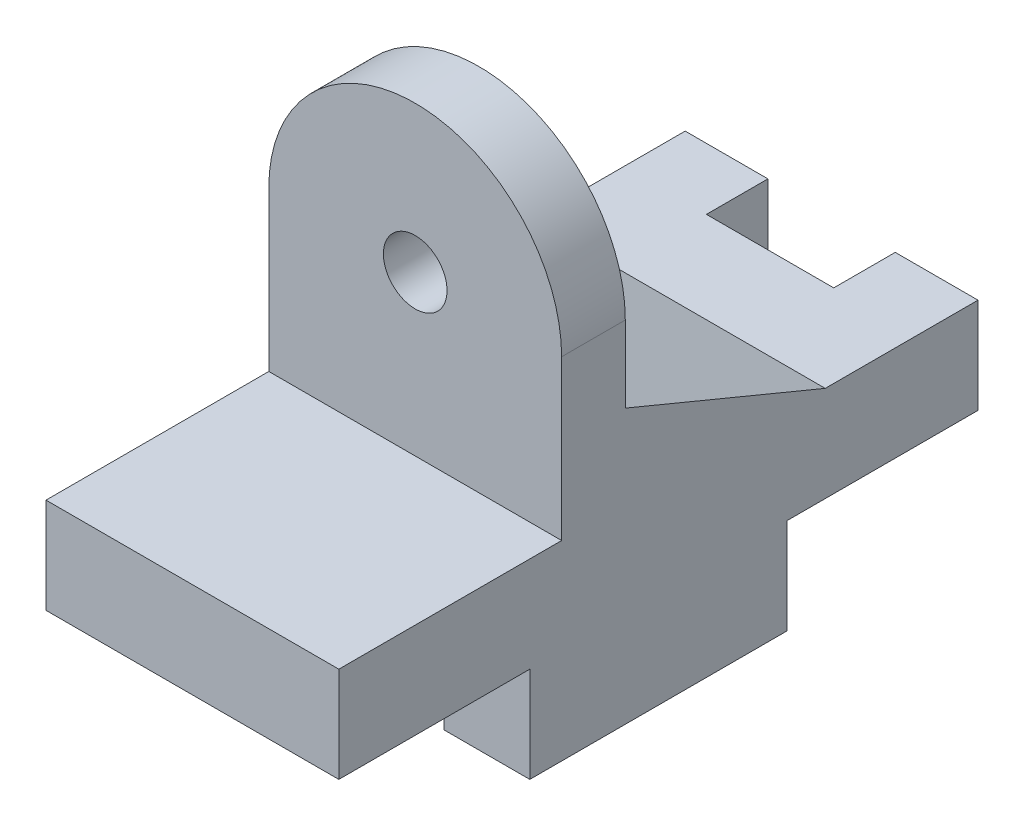
ISO-10303-21;
HEADER;
FILE_DESCRIPTION(('STEP AP214'),'2;1');
FILE_NAME('part.step','',(''),(''),'','','');
FILE_SCHEMA(('AUTOMOTIVE_DESIGN { 1 0 10303 214 1 1 1 1 }'));
ENDSEC;
DATA;
#1=APPLICATION_CONTEXT('core data for automotive mechanical design processes');
#2=APPLICATION_PROTOCOL_DEFINITION('international standard','automotive_design',2000,#1);
#3=PRODUCT_CONTEXT('',#1,'mechanical');
#4=PRODUCT('Part','Part','',(#3));
#5=PRODUCT_RELATED_PRODUCT_CATEGORY('part','',(#4));
#6=PRODUCT_DEFINITION_FORMATION('','',#4);
#7=PRODUCT_DEFINITION_CONTEXT('part definition',#1,'design');
#8=PRODUCT_DEFINITION('design','',#6,#7);
#9=PRODUCT_DEFINITION_SHAPE('','',#8);
#10=(LENGTH_UNIT() NAMED_UNIT(*) SI_UNIT(.MILLI.,.METRE.));
#11=(NAMED_UNIT(*) PLANE_ANGLE_UNIT() SI_UNIT($,.RADIAN.));
#12=(NAMED_UNIT(*) SI_UNIT($,.STERADIAN.) SOLID_ANGLE_UNIT());
#13=UNCERTAINTY_MEASURE_WITH_UNIT(LENGTH_MEASURE(1.E-05),#10,'distance_accuracy_value','');
#14=(GEOMETRIC_REPRESENTATION_CONTEXT(3) GLOBAL_UNCERTAINTY_ASSIGNED_CONTEXT((#13)) GLOBAL_UNIT_ASSIGNED_CONTEXT((#10,
#11,#12)) REPRESENTATION_CONTEXT('',''));
#15=CARTESIAN_POINT('',(0.,0.,0.));
#16=DIRECTION('',(0.,0.,1.));
#17=DIRECTION('',(1.,0.,0.));
#18=AXIS2_PLACEMENT_3D('',#15,#16,#17);
#19=CARTESIAN_POINT('',(46.,-15.,20.2023099235515));
#20=DIRECTION('',(0.,0.,-1.));
#21=DIRECTION('',(0.,1.,0.));
#22=AXIS2_PLACEMENT_3D('',#19,#20,#21);
#23=PLANE('',#22);
#24=DIRECTION('',(-1.,0.,0.));
#25=VECTOR('',#24,1.);
#26=CARTESIAN_POINT('',(46.,-30.,20.2023099235515));
#27=LINE('',#26,#25);
#28=CARTESIAN_POINT('',(13.5,-30.,20.2023099235515));
#29=VERTEX_POINT('',#28);
#30=CARTESIAN_POINT('',(0.,-30.,20.2023099235515));
#31=VERTEX_POINT('',#30);
#32=EDGE_CURVE('E220',#29,#31,#27,.T.);
#33=ORIENTED_EDGE('',*,*,#32,.F.);
#34=DIRECTION('',(0.,1.,0.));
#35=VECTOR('',#34,1.);
#36=CARTESIAN_POINT('',(13.5,-15.,20.2023099235515));
#37=LINE('',#36,#35);
#38=CARTESIAN_POINT('',(13.5,-15.,20.2023099235515));
#39=VERTEX_POINT('',#38);
#40=EDGE_CURVE('E346',#29,#39,#37,.T.);
#41=ORIENTED_EDGE('',*,*,#40,.T.);
#42=DIRECTION('',(-1.,0.,0.));
#43=VECTOR('',#42,1.);
#44=CARTESIAN_POINT('',(46.,-15.,20.2023099235515));
#45=LINE('',#44,#43);
#46=CARTESIAN_POINT('',(0.,-15.,20.2023099235515));
#47=VERTEX_POINT('',#46);
#48=EDGE_CURVE('E221',#39,#47,#45,.T.);
#49=ORIENTED_EDGE('',*,*,#48,.T.);
#50=DIRECTION('',(0.,-1.,0.));
#51=VECTOR('',#50,1.);
#52=CARTESIAN_POINT('',(0.,-15.,20.2023099235515));
#53=LINE('',#52,#51);
#54=EDGE_CURVE('E270',#47,#31,#53,.T.);
#55=ORIENTED_EDGE('',*,*,#54,.T.);
#56=EDGE_LOOP('',(#33,#41,#49,#55));
#57=FACE_BOUND('',#56,.T.);
#58=ADVANCED_FACE('F41',(#57),#23,.F.);
#59=CARTESIAN_POINT('',(46.,-30.,-20.2023099235515));
#60=DIRECTION('',(0.,1.,0.));
#61=DIRECTION('',(0.,0.,1.));
#62=AXIS2_PLACEMENT_3D('',#59,#60,#61);
#63=PLANE('',#62);
#64=DIRECTION('',(-1.,0.,0.));
#65=VECTOR('',#64,1.);
#66=CARTESIAN_POINT('',(46.,-30.,-20.2023099235515));
#67=LINE('',#66,#65);
#68=CARTESIAN_POINT('',(13.5,-30.,-20.2023099235515));
#69=VERTEX_POINT('',#68);
#70=CARTESIAN_POINT('',(0.,-30.,-20.2023099235515));
#71=VERTEX_POINT('',#70);
#72=EDGE_CURVE('E209',#69,#71,#67,.T.);
#73=ORIENTED_EDGE('',*,*,#72,.F.);
#74=DIRECTION('',(0.,0.,1.));
#75=VECTOR('',#74,1.);
#76=CARTESIAN_POINT('',(13.5,-30.,-20.2023099235515));
#77=LINE('',#76,#75);
#78=EDGE_CURVE('E351',#69,#29,#77,.T.);
#79=ORIENTED_EDGE('',*,*,#78,.T.);
#80=ORIENTED_EDGE('',*,*,#32,.T.);
#81=DIRECTION('',(0.,0.,-1.));
#82=VECTOR('',#81,1.);
#83=CARTESIAN_POINT('',(0.,-30.,-20.2023099235515));
#84=LINE('',#83,#82);
#85=EDGE_CURVE('E267',#31,#71,#84,.T.);
#86=ORIENTED_EDGE('',*,*,#85,.T.);
#87=EDGE_LOOP('',(#73,#79,#80,#86));
#88=FACE_BOUND('',#87,.T.);
#89=ADVANCED_FACE('F401',(#88),#63,.F.);
#90=CARTESIAN_POINT('',(46.,-15.,-20.2023099235515));
#91=DIRECTION('',(0.,0.,1.));
#92=DIRECTION('',(1.,0.,0.));
#93=AXIS2_PLACEMENT_3D('',#90,#91,#92);
#94=PLANE('',#93);
#95=DIRECTION('',(-1.,0.,0.));
#96=VECTOR('',#95,1.);
#97=CARTESIAN_POINT('',(46.,-15.,-20.2023099235515));
#98=LINE('',#97,#96);
#99=CARTESIAN_POINT('',(13.5,-15.,-20.2023099235515));
#100=VERTEX_POINT('',#99);
#101=CARTESIAN_POINT('',(0.,-15.,-20.2023099235515));
#102=VERTEX_POINT('',#101);
#103=EDGE_CURVE('E208',#100,#102,#98,.T.);
#104=ORIENTED_EDGE('',*,*,#103,.F.);
#105=DIRECTION('',(0.,1.,0.));
#106=VECTOR('',#105,1.);
#107=CARTESIAN_POINT('',(13.5,-15.,-20.2023099235515));
#108=LINE('',#107,#106);
#109=EDGE_CURVE('E194',#69,#100,#108,.T.);
#110=ORIENTED_EDGE('',*,*,#109,.F.);
#111=ORIENTED_EDGE('',*,*,#72,.T.);
#112=DIRECTION('',(0.,1.,0.));
#113=VECTOR('',#112,1.);
#114=CARTESIAN_POINT('',(0.,-15.,-20.2023099235515));
#115=LINE('',#114,#113);
#116=EDGE_CURVE('E264',#71,#102,#115,.T.);
#117=ORIENTED_EDGE('',*,*,#116,.T.);
#118=EDGE_LOOP('',(#104,#110,#111,#117));
#119=FACE_BOUND('',#118,.T.);
#120=ADVANCED_FACE('F364',(#119),#94,.F.);
#121=CARTESIAN_POINT('',(46.,0.,-50.2023099235515));
#122=DIRECTION('',(0.,0.,1.));
#123=DIRECTION('',(1.,0.,0.));
#124=AXIS2_PLACEMENT_3D('',#121,#122,#123);
#125=PLANE('',#124);
#126=DIRECTION('',(-1.,0.,0.));
#127=VECTOR('',#126,1.);
#128=CARTESIAN_POINT('',(46.,0.,-50.2023099235515));
#129=LINE('',#128,#127);
#130=CARTESIAN_POINT('',(13.,0.,-50.2023099235515));
#131=VERTEX_POINT('',#130);
#132=CARTESIAN_POINT('',(0.,0.,-50.2023099235515));
#133=VERTEX_POINT('',#132);
#134=EDGE_CURVE('E235',#131,#133,#129,.T.);
#135=ORIENTED_EDGE('',*,*,#134,.F.);
#136=DIRECTION('',(0.,-1.,0.));
#137=VECTOR('',#136,1.);
#138=CARTESIAN_POINT('',(13.,0.,-50.2023099235515));
#139=LINE('',#138,#137);
#140=CARTESIAN_POINT('',(13.,-15.,-50.2023099235515));
#141=VERTEX_POINT('',#140);
#142=EDGE_CURVE('E47',#131,#141,#139,.T.);
#143=ORIENTED_EDGE('',*,*,#142,.T.);
#144=DIRECTION('',(-1.,0.,0.));
#145=VECTOR('',#144,1.);
#146=CARTESIAN_POINT('',(46.,-15.,-50.2023099235515));
#147=LINE('',#146,#145);
#148=CARTESIAN_POINT('',(0.,-15.,-50.2023099235515));
#149=VERTEX_POINT('',#148);
#150=EDGE_CURVE('E229',#141,#149,#147,.T.);
#151=ORIENTED_EDGE('',*,*,#150,.T.);
#152=DIRECTION('',(0.,1.,0.));
#153=VECTOR('',#152,1.);
#154=CARTESIAN_POINT('',(0.,0.,-50.2023099235515));
#155=LINE('',#154,#153);
#156=EDGE_CURVE('E263',#149,#133,#155,.T.);
#157=ORIENTED_EDGE('',*,*,#156,.T.);
#158=EDGE_LOOP('',(#135,#143,#151,#157));
#159=FACE_BOUND('',#158,.T.);
#160=ADVANCED_FACE('F226',(#159),#125,.F.);
#161=CARTESIAN_POINT('',(46.,0.,-50.2023099235515));
#162=DIRECTION('',(0.,-1.,0.));
#163=DIRECTION('',(0.,0.,-1.));
#164=AXIS2_PLACEMENT_3D('',#161,#162,#163);
#165=PLANE('',#164);
#166=DIRECTION('',(1.,0.,0.));
#167=VECTOR('',#166,1.);
#168=CARTESIAN_POINT('',(33.,0.,-40.5407293133356));
#169=LINE('',#168,#167);
#170=CARTESIAN_POINT('',(13.,0.,-40.5407293133356));
#171=VERTEX_POINT('',#170);
#172=CARTESIAN_POINT('',(33.,0.,-40.5407293133356));
#173=VERTEX_POINT('',#172);
#174=EDGE_CURVE('E344',#171,#173,#169,.T.);
#175=ORIENTED_EDGE('',*,*,#174,.F.);
#176=DIRECTION('',(0.,0.,1.));
#177=VECTOR('',#176,1.);
#178=CARTESIAN_POINT('',(13.,0.,-59.8638905337673));
#179=LINE('',#178,#177);
#180=EDGE_CURVE('E348',#131,#171,#179,.T.);
#181=ORIENTED_EDGE('',*,*,#180,.F.);
#182=ORIENTED_EDGE('',*,*,#134,.T.);
#183=DIRECTION('',(0.,0.,1.));
#184=VECTOR('',#183,1.);
#185=CARTESIAN_POINT('',(0.,0.,-50.2023099235515));
#186=LINE('',#185,#184);
#187=CARTESIAN_POINT('',(0.,0.,-26.2023099235514));
#188=VERTEX_POINT('',#187);
#189=EDGE_CURVE('E259',#133,#188,#186,.T.);
#190=ORIENTED_EDGE('',*,*,#189,.T.);
#191=DIRECTION('',(-1.,0.,0.));
#192=VECTOR('',#191,1.);
#193=CARTESIAN_POINT('',(46.,0.,-26.2023099235515));
#194=LINE('',#193,#192);
#195=CARTESIAN_POINT('',(46.,0.,-26.2023099235514));
#196=VERTEX_POINT('',#195);
#197=EDGE_CURVE('E304',#196,#188,#194,.T.);
#198=ORIENTED_EDGE('',*,*,#197,.F.);
#199=DIRECTION('',(0.,0.,1.));
#200=VECTOR('',#199,1.);
#201=CARTESIAN_POINT('',(46.,0.,-50.2023099235515));
#202=LINE('',#201,#200);
#203=CARTESIAN_POINT('',(46.,0.,-50.2023099235515));
#204=VERTEX_POINT('',#203);
#205=EDGE_CURVE('E279',#204,#196,#202,.T.);
#206=ORIENTED_EDGE('',*,*,#205,.F.);
#207=CARTESIAN_POINT('',(33.,0.,-50.2023099235515));
#208=VERTEX_POINT('',#207);
#209=EDGE_CURVE('E241',#204,#208,#129,.T.);
#210=ORIENTED_EDGE('',*,*,#209,.T.);
#211=DIRECTION('',(0.,0.,-1.));
#212=VECTOR('',#211,1.);
#213=CARTESIAN_POINT('',(33.,0.,-59.8638905337673));
#214=LINE('',#213,#212);
#215=EDGE_CURVE('E61',#173,#208,#214,.T.);
#216=ORIENTED_EDGE('',*,*,#215,.F.);
#217=EDGE_LOOP('',(#175,#181,#182,#190,#198,#206,#210,#216));
#218=FACE_BOUND('',#217,.T.);
#219=ADVANCED_FACE('F375',(#218),#165,.F.);
#220=CARTESIAN_POINT('',(46.,0.,5.20230992355147));
#221=DIRECTION('',(0.,0.,1.));
#222=DIRECTION('',(1.,0.,0.));
#223=AXIS2_PLACEMENT_3D('',#220,#221,#222);
#224=PLANE('',#223);
#225=CARTESIAN_POINT('',(23.,25.,5.20230992355147));
#226=DIRECTION('',(0.,0.,-1.));
#227=DIRECTION('',(-1.,0.,0.));
#228=AXIS2_PLACEMENT_3D('',#225,#226,#227);
#229=CIRCLE('',#228,5.);
#230=CARTESIAN_POINT('',(18.,25.,5.20230992355147));
#231=VERTEX_POINT('',#230);
#232=EDGE_CURVE('E329',#231,#231,#229,.T.);
#233=ORIENTED_EDGE('',*,*,#232,.F.);
#234=EDGE_LOOP('',(#233));
#235=FACE_BOUND('',#234,.T.);
#236=DIRECTION('',(-1.,0.,0.));
#237=VECTOR('',#236,1.);
#238=CARTESIAN_POINT('',(46.,13.0151880614219,5.20230992355147));
#239=LINE('',#238,#237);
#240=CARTESIAN_POINT('',(46.,13.0151880614219,5.20230992355147));
#241=VERTEX_POINT('',#240);
#242=CARTESIAN_POINT('',(0.,13.0151880614219,5.20230992355147));
#243=VERTEX_POINT('',#242);
#244=EDGE_CURVE('E313',#241,#243,#239,.T.);
#245=ORIENTED_EDGE('',*,*,#244,.T.);
#246=DIRECTION('',(0.,1.,0.));
#247=VECTOR('',#246,1.);
#248=CARTESIAN_POINT('',(0.,0.,5.20230992355147));
#249=LINE('',#248,#247);
#250=CARTESIAN_POINT('',(0.,25.,5.20230992355147));
#251=VERTEX_POINT('',#250);
#252=EDGE_CURVE('E305',#243,#251,#249,.T.);
#253=ORIENTED_EDGE('',*,*,#252,.T.);
#254=CARTESIAN_POINT('',(23.,25.,5.20230992355147));
#255=DIRECTION('',(0.,0.,-1.));
#256=DIRECTION('',(-1.,0.,0.));
#257=AXIS2_PLACEMENT_3D('',#254,#255,#256);
#258=CIRCLE('',#257,23.);
#259=CARTESIAN_POINT('',(46.,25.,5.20230992355147));
#260=VERTEX_POINT('',#259);
#261=EDGE_CURVE('E321',#251,#260,#258,.T.);
#262=ORIENTED_EDGE('',*,*,#261,.T.);
#263=DIRECTION('',(0.,1.,0.));
#264=VECTOR('',#263,1.);
#265=CARTESIAN_POINT('',(46.,0.,5.20230992355147));
#266=LINE('',#265,#264);
#267=EDGE_CURVE('E296',#241,#260,#266,.T.);
#268=ORIENTED_EDGE('',*,*,#267,.F.);
#269=EDGE_LOOP('',(#245,#253,#262,#268));
#270=FACE_BOUND('',#269,.T.);
#271=ADVANCED_FACE('F412',(#235,#270),#224,.F.);
#272=CARTESIAN_POINT('',(46.,-15.,20.2023099235515));
#273=VERTEX_POINT('',#272);
#274=CARTESIAN_POINT('',(32.5,-15.,20.2023099235515));
#275=VERTEX_POINT('',#274);
#276=EDGE_CURVE('E222',#273,#275,#45,.T.);
#277=ORIENTED_EDGE('',*,*,#276,.T.);
#278=DIRECTION('',(0.,-1.,0.));
#279=VECTOR('',#278,1.);
#280=CARTESIAN_POINT('',(32.5,-15.,20.2023099235515));
#281=LINE('',#280,#279);
#282=CARTESIAN_POINT('',(32.5,-30.,20.2023099235515));
#283=VERTEX_POINT('',#282);
#284=EDGE_CURVE('E186',#275,#283,#281,.T.);
#285=ORIENTED_EDGE('',*,*,#284,.T.);
#286=CARTESIAN_POINT('',(46.,-30.,20.2023099235515));
#287=VERTEX_POINT('',#286);
#288=EDGE_CURVE('E216',#287,#283,#27,.T.);
#289=ORIENTED_EDGE('',*,*,#288,.F.);
#290=DIRECTION('',(0.,-1.,0.));
#291=VECTOR('',#290,1.);
#292=CARTESIAN_POINT('',(46.,-15.,20.2023099235515));
#293=LINE('',#292,#291);
#294=EDGE_CURVE('E288',#273,#287,#293,.T.);
#295=ORIENTED_EDGE('',*,*,#294,.F.);
#296=EDGE_LOOP('',(#277,#285,#289,#295));
#297=FACE_BOUND('',#296,.T.);
#298=ADVANCED_FACE('F43',(#297),#23,.F.);
#299=ORIENTED_EDGE('',*,*,#288,.T.);
#300=DIRECTION('',(0.,0.,-1.));
#301=VECTOR('',#300,1.);
#302=CARTESIAN_POINT('',(32.5,-30.,-20.2023099235515));
#303=LINE('',#302,#301);
#304=CARTESIAN_POINT('',(32.5,-30.,-20.2023099235515));
#305=VERTEX_POINT('',#304);
#306=EDGE_CURVE('E355',#283,#305,#303,.T.);
#307=ORIENTED_EDGE('',*,*,#306,.T.);
#308=CARTESIAN_POINT('',(46.,-30.,-20.2023099235515));
#309=VERTEX_POINT('',#308);
#310=EDGE_CURVE('E204',#309,#305,#67,.T.);
#311=ORIENTED_EDGE('',*,*,#310,.F.);
#312=DIRECTION('',(0.,0.,-1.));
#313=VECTOR('',#312,1.);
#314=CARTESIAN_POINT('',(46.,-30.,-20.2023099235515));
#315=LINE('',#314,#313);
#316=EDGE_CURVE('E287',#287,#309,#315,.T.);
#317=ORIENTED_EDGE('',*,*,#316,.F.);
#318=EDGE_LOOP('',(#299,#307,#311,#317));
#319=FACE_BOUND('',#318,.T.);
#320=ADVANCED_FACE('F390',(#319),#63,.F.);
#321=ORIENTED_EDGE('',*,*,#310,.T.);
#322=DIRECTION('',(0.,-1.,0.));
#323=VECTOR('',#322,1.);
#324=CARTESIAN_POINT('',(32.5,-32.214795118551,-20.2023099235515));
#325=LINE('',#324,#323);
#326=CARTESIAN_POINT('',(32.5,-15.,-20.2023099235515));
#327=VERTEX_POINT('',#326);
#328=EDGE_CURVE('E187',#327,#305,#325,.T.);
#329=ORIENTED_EDGE('',*,*,#328,.F.);
#330=CARTESIAN_POINT('',(46.,-15.,-20.2023099235515));
#331=VERTEX_POINT('',#330);
#332=EDGE_CURVE('E197',#331,#327,#98,.T.);
#333=ORIENTED_EDGE('',*,*,#332,.F.);
#334=DIRECTION('',(0.,1.,0.));
#335=VECTOR('',#334,1.);
#336=CARTESIAN_POINT('',(46.,-15.,-20.2023099235515));
#337=LINE('',#336,#335);
#338=EDGE_CURVE('E282',#309,#331,#337,.T.);
#339=ORIENTED_EDGE('',*,*,#338,.F.);
#340=EDGE_LOOP('',(#321,#329,#333,#339));
#341=FACE_BOUND('',#340,.T.);
#342=ADVANCED_FACE('F196',(#341),#94,.F.);
#343=CARTESIAN_POINT('',(46.,-15.,-50.2023099235515));
#344=DIRECTION('',(0.,1.,0.));
#345=DIRECTION('',(0.,0.,1.));
#346=AXIS2_PLACEMENT_3D('',#343,#344,#345);
#347=PLANE('',#346);
#348=ORIENTED_EDGE('',*,*,#150,.F.);
#349=DIRECTION('',(0.,0.,1.));
#350=VECTOR('',#349,1.);
#351=CARTESIAN_POINT('',(13.,-15.,-50.2023099235515));
#352=LINE('',#351,#350);
#353=CARTESIAN_POINT('',(13.,-15.,-40.5407293133356));
#354=VERTEX_POINT('',#353);
#355=EDGE_CURVE('E240',#141,#354,#352,.T.);
#356=ORIENTED_EDGE('',*,*,#355,.T.);
#357=DIRECTION('',(1.,0.,0.));
#358=VECTOR('',#357,1.);
#359=CARTESIAN_POINT('',(46.,-15.,-40.5407293133356));
#360=LINE('',#359,#358);
#361=CARTESIAN_POINT('',(33.,-15.,-40.5407293133356));
#362=VERTEX_POINT('',#361);
#363=EDGE_CURVE('E11',#354,#362,#360,.T.);
#364=ORIENTED_EDGE('',*,*,#363,.T.);
#365=DIRECTION('',(0.,0.,-1.));
#366=VECTOR('',#365,1.);
#367=CARTESIAN_POINT('',(33.,-15.,-50.2023099235515));
#368=LINE('',#367,#366);
#369=CARTESIAN_POINT('',(33.,-15.,-50.2023099235515));
#370=VERTEX_POINT('',#369);
#371=EDGE_CURVE('E335',#362,#370,#368,.T.);
#372=ORIENTED_EDGE('',*,*,#371,.T.);
#373=CARTESIAN_POINT('',(46.,-15.,-50.2023099235515));
#374=VERTEX_POINT('',#373);
#375=EDGE_CURVE('E214',#374,#370,#147,.T.);
#376=ORIENTED_EDGE('',*,*,#375,.F.);
#377=DIRECTION('',(0.,0.,-1.));
#378=VECTOR('',#377,1.);
#379=CARTESIAN_POINT('',(46.,-15.,-50.2023099235515));
#380=LINE('',#379,#378);
#381=EDGE_CURVE('E206',#331,#374,#380,.T.);
#382=ORIENTED_EDGE('',*,*,#381,.F.);
#383=ORIENTED_EDGE('',*,*,#332,.T.);
#384=DIRECTION('',(0.,0.,-1.));
#385=VECTOR('',#384,1.);
#386=CARTESIAN_POINT('',(32.5,-15.,60.7976900764485));
#387=LINE('',#386,#385);
#388=EDGE_CURVE('E182',#275,#327,#387,.T.);
#389=ORIENTED_EDGE('',*,*,#388,.F.);
#390=ORIENTED_EDGE('',*,*,#276,.F.);
#391=DIRECTION('',(0.,0.,-1.));
#392=VECTOR('',#391,1.);
#393=CARTESIAN_POINT('',(46.,-15.,50.2023099235515));
#394=LINE('',#393,#392);
#395=CARTESIAN_POINT('',(46.,-15.,50.2023099235515));
#396=VERTEX_POINT('',#395);
#397=EDGE_CURVE('E260',#396,#273,#394,.T.);
#398=ORIENTED_EDGE('',*,*,#397,.F.);
#399=DIRECTION('',(-1.,0.,0.));
#400=VECTOR('',#399,1.);
#401=CARTESIAN_POINT('',(46.,-15.,50.2023099235515));
#402=LINE('',#401,#400);
#403=CARTESIAN_POINT('',(0.,-15.,50.2023099235515));
#404=VERTEX_POINT('',#403);
#405=EDGE_CURVE('E252',#396,#404,#402,.T.);
#406=ORIENTED_EDGE('',*,*,#405,.T.);
#407=DIRECTION('',(0.,0.,-1.));
#408=VECTOR('',#407,1.);
#409=CARTESIAN_POINT('',(0.,-15.,50.2023099235515));
#410=LINE('',#409,#408);
#411=EDGE_CURVE('E271',#404,#47,#410,.T.);
#412=ORIENTED_EDGE('',*,*,#411,.T.);
#413=ORIENTED_EDGE('',*,*,#48,.F.);
#414=DIRECTION('',(0.,0.,-1.));
#415=VECTOR('',#414,1.);
#416=CARTESIAN_POINT('',(13.5,-15.,60.7976900764485));
#417=LINE('',#416,#415);
#418=EDGE_CURVE('E57',#39,#100,#417,.T.);
#419=ORIENTED_EDGE('',*,*,#418,.T.);
#420=ORIENTED_EDGE('',*,*,#103,.T.);
#421=DIRECTION('',(0.,0.,-1.));
#422=VECTOR('',#421,1.);
#423=CARTESIAN_POINT('',(0.,-15.,-50.2023099235515));
#424=LINE('',#423,#422);
#425=EDGE_CURVE('E237',#102,#149,#424,.T.);
#426=ORIENTED_EDGE('',*,*,#425,.T.);
#427=EDGE_LOOP('',(#348,#356,#364,#372,#376,#382,#383,#389,#390,#398,#406,#412,#413,#419,#420,#426));
#428=FACE_BOUND('',#427,.T.);
#429=ADVANCED_FACE('F207',(#428),#347,.F.);
#430=ORIENTED_EDGE('',*,*,#375,.T.);
#431=DIRECTION('',(0.,1.,0.));
#432=VECTOR('',#431,1.);
#433=CARTESIAN_POINT('',(33.,0.,-50.2023099235515));
#434=LINE('',#433,#432);
#435=EDGE_CURVE('E223',#370,#208,#434,.T.);
#436=ORIENTED_EDGE('',*,*,#435,.T.);
#437=ORIENTED_EDGE('',*,*,#209,.F.);
#438=DIRECTION('',(0.,1.,0.));
#439=VECTOR('',#438,1.);
#440=CARTESIAN_POINT('',(46.,0.,-50.2023099235515));
#441=LINE('',#440,#439);
#442=EDGE_CURVE('E285',#374,#204,#441,.T.);
#443=ORIENTED_EDGE('',*,*,#442,.F.);
#444=EDGE_LOOP('',(#430,#436,#437,#443));
#445=FACE_BOUND('',#444,.T.);
#446=ADVANCED_FACE('F379',(#445),#125,.F.);
#447=CARTESIAN_POINT('',(46.,0.,15.2023099235515));
#448=VERTEX_POINT('',#447);
#449=CARTESIAN_POINT('',(46.,0.,50.2023099235515));
#450=VERTEX_POINT('',#449);
#451=EDGE_CURVE('E283',#448,#450,#202,.T.);
#452=ORIENTED_EDGE('',*,*,#451,.F.);
#453=DIRECTION('',(-1.,0.,0.));
#454=VECTOR('',#453,1.);
#455=CARTESIAN_POINT('',(46.,0.,15.2023099235515));
#456=LINE('',#455,#454);
#457=CARTESIAN_POINT('',(0.,0.,15.2023099235515));
#458=VERTEX_POINT('',#457);
#459=EDGE_CURVE('E277',#448,#458,#456,.T.);
#460=ORIENTED_EDGE('',*,*,#459,.T.);
#461=CARTESIAN_POINT('',(0.,0.,50.2023099235515));
#462=VERTEX_POINT('',#461);
#463=EDGE_CURVE('E258',#458,#462,#186,.T.);
#464=ORIENTED_EDGE('',*,*,#463,.T.);
#465=DIRECTION('',(-1.,0.,0.));
#466=VECTOR('',#465,1.);
#467=CARTESIAN_POINT('',(46.,0.,50.2023099235515));
#468=LINE('',#467,#466);
#469=EDGE_CURVE('E250',#450,#462,#468,.T.);
#470=ORIENTED_EDGE('',*,*,#469,.F.);
#471=EDGE_LOOP('',(#452,#460,#464,#470));
#472=FACE_BOUND('',#471,.T.);
#473=ADVANCED_FACE('F430',(#472),#165,.F.);
#474=CARTESIAN_POINT('',(46.,0.,50.2023099235515));
#475=DIRECTION('',(0.,0.,-1.));
#476=DIRECTION('',(-1.,0.,0.));
#477=AXIS2_PLACEMENT_3D('',#474,#475,#476);
#478=PLANE('',#477);
#479=DIRECTION('',(0.,-1.,0.));
#480=VECTOR('',#479,1.);
#481=CARTESIAN_POINT('',(0.,0.,50.2023099235515));
#482=LINE('',#481,#480);
#483=EDGE_CURVE('E251',#462,#404,#482,.T.);
#484=ORIENTED_EDGE('',*,*,#483,.T.);
#485=ORIENTED_EDGE('',*,*,#405,.F.);
#486=DIRECTION('',(0.,-1.,0.));
#487=VECTOR('',#486,1.);
#488=CARTESIAN_POINT('',(46.,0.,50.2023099235515));
#489=LINE('',#488,#487);
#490=EDGE_CURVE('E254',#450,#396,#489,.T.);
#491=ORIENTED_EDGE('',*,*,#490,.F.);
#492=ORIENTED_EDGE('',*,*,#469,.T.);
#493=EDGE_LOOP('',(#484,#485,#491,#492));
#494=FACE_BOUND('',#493,.T.);
#495=ADVANCED_FACE('F392',(#494),#478,.F.);
#496=CARTESIAN_POINT('',(46.,0.,0.));
#497=DIRECTION('',(-1.,0.,0.));
#498=DIRECTION('',(0.,0.,1.));
#499=AXIS2_PLACEMENT_3D('',#496,#497,#498);
#500=PLANE('',#499);
#501=ORIENTED_EDGE('',*,*,#205,.T.);
#502=DIRECTION('',(0.,0.382858395638294,0.923807040939433));
#503=VECTOR('',#502,1.);
#504=CARTESIAN_POINT('',(46.,13.0151880614219,5.20230992355147));
#505=LINE('',#504,#503);
#506=EDGE_CURVE('E320',#196,#241,#505,.T.);
#507=ORIENTED_EDGE('',*,*,#506,.T.);
#508=ORIENTED_EDGE('',*,*,#267,.T.);
#509=DIRECTION('',(0.,0.,1.));
#510=VECTOR('',#509,1.);
#511=CARTESIAN_POINT('',(46.,25.,5.20230992355147));
#512=LINE('',#511,#510);
#513=CARTESIAN_POINT('',(46.,25.,15.2023099235515));
#514=VERTEX_POINT('',#513);
#515=EDGE_CURVE('E310',#260,#514,#512,.T.);
#516=ORIENTED_EDGE('',*,*,#515,.T.);
#517=DIRECTION('',(0.,-1.,0.));
#518=VECTOR('',#517,1.);
#519=CARTESIAN_POINT('',(46.,0.,15.2023099235515));
#520=LINE('',#519,#518);
#521=EDGE_CURVE('E294',#514,#448,#520,.T.);
#522=ORIENTED_EDGE('',*,*,#521,.T.);
#523=ORIENTED_EDGE('',*,*,#451,.T.);
#524=ORIENTED_EDGE('',*,*,#490,.T.);
#525=ORIENTED_EDGE('',*,*,#397,.T.);
#526=ORIENTED_EDGE('',*,*,#294,.T.);
#527=ORIENTED_EDGE('',*,*,#316,.T.);
#528=ORIENTED_EDGE('',*,*,#338,.T.);
#529=ORIENTED_EDGE('',*,*,#381,.T.);
#530=ORIENTED_EDGE('',*,*,#442,.T.);
#531=EDGE_LOOP('',(#501,#507,#508,#516,#522,#523,#524,#525,#526,#527,#528,#529,#530));
#532=FACE_BOUND('',#531,.T.);
#533=ADVANCED_FACE('F385',(#532),#500,.F.);
#534=CARTESIAN_POINT('',(0.,0.,0.));
#535=DIRECTION('',(-1.,0.,0.));
#536=DIRECTION('',(0.,0.,1.));
#537=AXIS2_PLACEMENT_3D('',#534,#535,#536);
#538=PLANE('',#537);
#539=DIRECTION('',(0.,0.382858395638294,0.923807040939433));
#540=VECTOR('',#539,1.);
#541=CARTESIAN_POINT('',(0.,13.0151880614219,5.20230992355147));
#542=LINE('',#541,#540);
#543=EDGE_CURVE('E319',#188,#243,#542,.T.);
#544=ORIENTED_EDGE('',*,*,#543,.F.);
#545=ORIENTED_EDGE('',*,*,#189,.F.);
#546=ORIENTED_EDGE('',*,*,#156,.F.);
#547=ORIENTED_EDGE('',*,*,#425,.F.);
#548=ORIENTED_EDGE('',*,*,#116,.F.);
#549=ORIENTED_EDGE('',*,*,#85,.F.);
#550=ORIENTED_EDGE('',*,*,#54,.F.);
#551=ORIENTED_EDGE('',*,*,#411,.F.);
#552=ORIENTED_EDGE('',*,*,#483,.F.);
#553=ORIENTED_EDGE('',*,*,#463,.F.);
#554=DIRECTION('',(0.,-1.,0.));
#555=VECTOR('',#554,1.);
#556=CARTESIAN_POINT('',(0.,0.,15.2023099235515));
#557=LINE('',#556,#555);
#558=CARTESIAN_POINT('',(0.,25.,15.2023099235515));
#559=VERTEX_POINT('',#558);
#560=EDGE_CURVE('E298',#559,#458,#557,.T.);
#561=ORIENTED_EDGE('',*,*,#560,.F.);
#562=DIRECTION('',(0.,0.,1.));
#563=VECTOR('',#562,1.);
#564=CARTESIAN_POINT('',(0.,25.,5.20230992355147));
#565=LINE('',#564,#563);
#566=EDGE_CURVE('E299',#251,#559,#565,.T.);
#567=ORIENTED_EDGE('',*,*,#566,.F.);
#568=ORIENTED_EDGE('',*,*,#252,.F.);
#569=EDGE_LOOP('',(#544,#545,#546,#547,#548,#549,#550,#551,#552,#553,#561,#567,#568));
#570=FACE_BOUND('',#569,.T.);
#571=ADVANCED_FACE('F367',(#570),#538,.T.);
#572=CARTESIAN_POINT('',(46.,0.,15.2023099235515));
#573=DIRECTION('',(0.,0.,-1.));
#574=DIRECTION('',(-1.,0.,0.));
#575=AXIS2_PLACEMENT_3D('',#572,#573,#574);
#576=PLANE('',#575);
#577=CARTESIAN_POINT('',(23.,25.,15.2023099235515));
#578=DIRECTION('',(0.,0.,-1.));
#579=DIRECTION('',(-1.,0.,0.));
#580=AXIS2_PLACEMENT_3D('',#577,#578,#579);
#581=CIRCLE('',#580,5.);
#582=CARTESIAN_POINT('',(18.,25.,15.2023099235515));
#583=VERTEX_POINT('',#582);
#584=EDGE_CURVE('E330',#583,#583,#581,.T.);
#585=ORIENTED_EDGE('',*,*,#584,.T.);
#586=EDGE_LOOP('',(#585));
#587=FACE_BOUND('',#586,.T.);
#588=ORIENTED_EDGE('',*,*,#560,.T.);
#589=ORIENTED_EDGE('',*,*,#459,.F.);
#590=ORIENTED_EDGE('',*,*,#521,.F.);
#591=CARTESIAN_POINT('',(23.,25.,15.2023099235515));
#592=DIRECTION('',(0.,0.,-1.));
#593=DIRECTION('',(-1.,0.,0.));
#594=AXIS2_PLACEMENT_3D('',#591,#592,#593);
#595=CIRCLE('',#594,23.);
#596=EDGE_CURVE('E322',#559,#514,#595,.T.);
#597=ORIENTED_EDGE('',*,*,#596,.F.);
#598=EDGE_LOOP('',(#588,#589,#590,#597));
#599=FACE_BOUND('',#598,.T.);
#600=ADVANCED_FACE('F435',(#587,#599),#576,.F.);
#601=CARTESIAN_POINT('',(46.,13.0151880614219,5.20230992355147));
#602=DIRECTION('',(0.,-0.923807040939433,0.382858395638294));
#603=DIRECTION('',(0.,-0.382858395638294,-0.923807040939433));
#604=AXIS2_PLACEMENT_3D('',#601,#602,#603);
#605=PLANE('',#604);
#606=ORIENTED_EDGE('',*,*,#543,.T.);
#607=ORIENTED_EDGE('',*,*,#244,.F.);
#608=ORIENTED_EDGE('',*,*,#506,.F.);
#609=ORIENTED_EDGE('',*,*,#197,.T.);
#610=EDGE_LOOP('',(#606,#607,#608,#609));
#611=FACE_BOUND('',#610,.T.);
#612=ADVANCED_FACE('F537',(#611),#605,.F.);
#613=CARTESIAN_POINT('',(23.,25.,15.2023099235515));
#614=DIRECTION('',(0.,0.,-1.));
#615=DIRECTION('',(-1.,0.,0.));
#616=AXIS2_PLACEMENT_3D('',#613,#614,#615);
#617=CYLINDRICAL_SURFACE('',#616,23.);
#618=ORIENTED_EDGE('',*,*,#261,.F.);
#619=ORIENTED_EDGE('',*,*,#566,.T.);
#620=ORIENTED_EDGE('',*,*,#596,.T.);
#621=ORIENTED_EDGE('',*,*,#515,.F.);
#622=EDGE_LOOP('',(#618,#619,#620,#621));
#623=FACE_BOUND('',#622,.T.);
#624=ADVANCED_FACE('F527',(#623),#617,.T.);
#625=CARTESIAN_POINT('',(23.,25.,15.2023099235515));
#626=DIRECTION('',(0.,0.,-1.));
#627=DIRECTION('',(-1.,0.,0.));
#628=AXIS2_PLACEMENT_3D('',#625,#626,#627);
#629=CYLINDRICAL_SURFACE('',#628,5.);
#630=ORIENTED_EDGE('',*,*,#584,.F.);
#631=EDGE_LOOP('',(#630));
#632=FACE_BOUND('',#631,.T.);
#633=ORIENTED_EDGE('',*,*,#232,.T.);
#634=EDGE_LOOP('',(#633));
#635=FACE_BOUND('',#634,.T.);
#636=ADVANCED_FACE('F515',(#632,#635),#629,.F.);
#637=CARTESIAN_POINT('',(33.,-19.,-40.5407293133356));
#638=DIRECTION('',(0.,0.,1.));
#639=DIRECTION('',(0.,-1.,0.));
#640=AXIS2_PLACEMENT_3D('',#637,#638,#639);
#641=PLANE('',#640);
#642=DIRECTION('',(0.,1.,0.));
#643=VECTOR('',#642,1.);
#644=CARTESIAN_POINT('',(13.,-19.,-40.5407293133356));
#645=LINE('',#644,#643);
#646=EDGE_CURVE('E339',#354,#171,#645,.T.);
#647=ORIENTED_EDGE('',*,*,#646,.T.);
#648=ORIENTED_EDGE('',*,*,#174,.T.);
#649=DIRECTION('',(0.,1.,0.));
#650=VECTOR('',#649,1.);
#651=CARTESIAN_POINT('',(33.,-19.,-40.5407293133356));
#652=LINE('',#651,#650);
#653=EDGE_CURVE('E336',#362,#173,#652,.T.);
#654=ORIENTED_EDGE('',*,*,#653,.F.);
#655=ORIENTED_EDGE('',*,*,#363,.F.);
#656=EDGE_LOOP('',(#647,#648,#654,#655));
#657=FACE_BOUND('',#656,.T.);
#658=ADVANCED_FACE('F376',(#657),#641,.F.);
#659=CARTESIAN_POINT('',(13.,-19.,-59.8638905337673));
#660=DIRECTION('',(-1.,0.,0.));
#661=DIRECTION('',(0.,0.,1.));
#662=AXIS2_PLACEMENT_3D('',#659,#660,#661);
#663=PLANE('',#662);
#664=ORIENTED_EDGE('',*,*,#142,.F.);
#665=ORIENTED_EDGE('',*,*,#180,.T.);
#666=ORIENTED_EDGE('',*,*,#646,.F.);
#667=ORIENTED_EDGE('',*,*,#355,.F.);
#668=EDGE_LOOP('',(#664,#665,#666,#667));
#669=FACE_BOUND('',#668,.T.);
#670=ADVANCED_FACE('F372',(#669),#663,.F.);
#671=CARTESIAN_POINT('',(33.,-19.,-59.8638905337673));
#672=DIRECTION('',(1.,0.,0.));
#673=DIRECTION('',(0.,0.,-1.));
#674=AXIS2_PLACEMENT_3D('',#671,#672,#673);
#675=PLANE('',#674);
#676=ORIENTED_EDGE('',*,*,#653,.T.);
#677=ORIENTED_EDGE('',*,*,#215,.T.);
#678=ORIENTED_EDGE('',*,*,#435,.F.);
#679=ORIENTED_EDGE('',*,*,#371,.F.);
#680=EDGE_LOOP('',(#676,#677,#678,#679));
#681=FACE_BOUND('',#680,.T.);
#682=ADVANCED_FACE('F464',(#681),#675,.F.);
#683=CARTESIAN_POINT('',(13.5,-15.,60.7976900764485));
#684=DIRECTION('',(-1.,0.,0.));
#685=DIRECTION('',(0.,0.,1.));
#686=AXIS2_PLACEMENT_3D('',#683,#684,#685);
#687=PLANE('',#686);
#688=ORIENTED_EDGE('',*,*,#78,.F.);
#689=ORIENTED_EDGE('',*,*,#109,.T.);
#690=ORIENTED_EDGE('',*,*,#418,.F.);
#691=ORIENTED_EDGE('',*,*,#40,.F.);
#692=EDGE_LOOP('',(#688,#689,#690,#691));
#693=FACE_BOUND('',#692,.T.);
#694=ADVANCED_FACE('F363',(#693),#687,.F.);
#695=CARTESIAN_POINT('',(32.5,-32.214795118551,60.7976900764485));
#696=DIRECTION('',(1.,0.,0.));
#697=DIRECTION('',(0.,0.,-1.));
#698=AXIS2_PLACEMENT_3D('',#695,#696,#697);
#699=PLANE('',#698);
#700=ORIENTED_EDGE('',*,*,#388,.T.);
#701=ORIENTED_EDGE('',*,*,#328,.T.);
#702=ORIENTED_EDGE('',*,*,#306,.F.);
#703=ORIENTED_EDGE('',*,*,#284,.F.);
#704=EDGE_LOOP('',(#700,#701,#702,#703));
#705=FACE_BOUND('',#704,.T.);
#706=ADVANCED_FACE('F184',(#705),#699,.F.);
#707=CLOSED_SHELL('',(#58,#89,#120,#160,#219,#271,#298,#320,#342,#429,#446,#473,#495,#533,#571,
#600,#612,#624,#636,#658,#670,#682,#694,#706));
#708=MANIFOLD_SOLID_BREP('B2',#707);
#709=ADVANCED_BREP_SHAPE_REPRESENTATION('',(#18,#708),#14);
#710=SHAPE_DEFINITION_REPRESENTATION(#9,#709);
ENDSEC;
END-ISO-10303-21;
